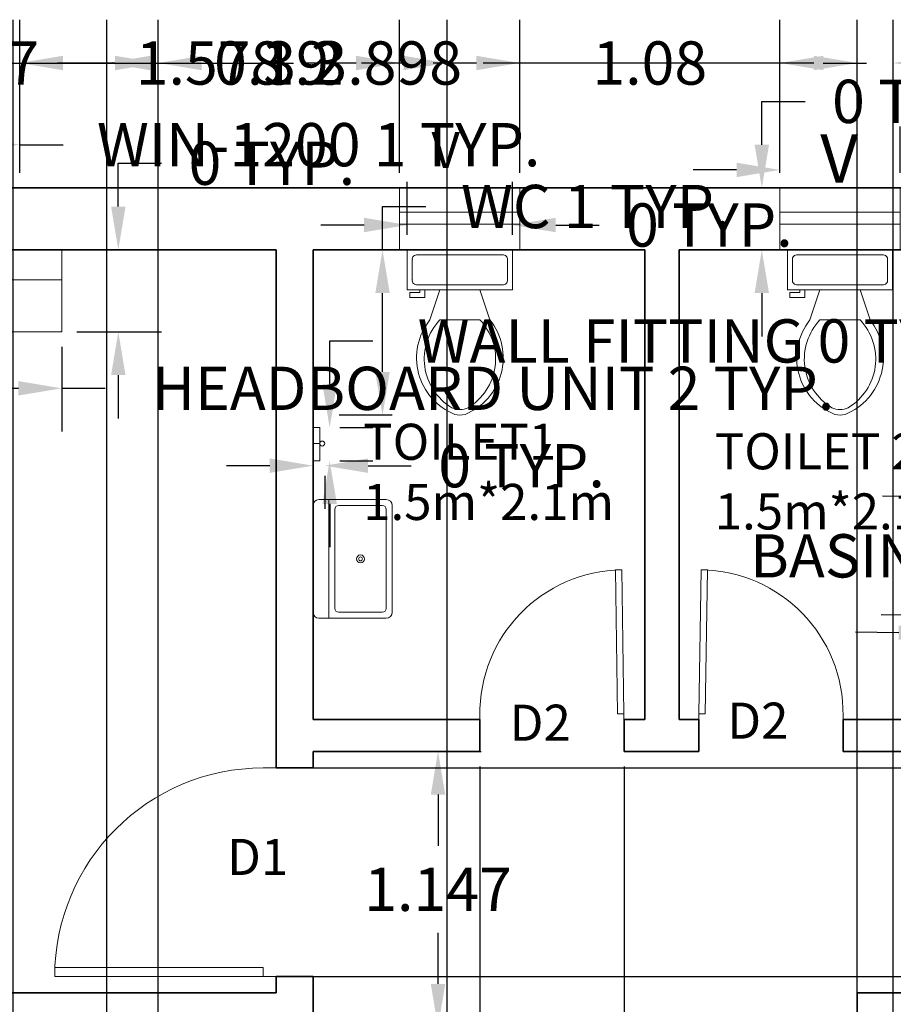
# Model space of a CAD drawing. Units: metres. Extents: x 1988.6 to 2001.1, y 2192 to 2202.5.
# Tile 4 of 6: x 1991.6 to 1995.3, y 2198.4 to 2202.5. Entities that reach past the tile are written whole.
import ezdxf

# ---------------------------------------------------------------- set-up
doc = ezdxf.new("R2010")
doc.units = ezdxf.units.M
for name, color, linetype, lineweight in [('A-ANNO-DIMS', 2, 'Continuous', 18), ('A-ANNO-TEXT', 7, 'Continuous', 18), ('A-AREA-IDEN', 7, 'Continuous', 18), ('A-DOOR', 3, 'Continuous', 18), ('A-FLOR-FIXT', 9, 'Continuous', 18), ('A-FURN', 9, 'Continuous', 15), ('A-GLAZ', 4, 'Continuous', 18), ('A-WALL', 7, 'Continuous', 35)]:
    doc.layers.add(name, color=color, linetype=linetype, lineweight=lineweight)
doc.styles.get("Standard").update_dxf_attribs({"font": 'arial.ttf'})
doc.dimstyles.get("Standard").update_dxf_attribs({"dimtxt": 0.18, "dimasz": 0.18, "dimexe": 0.18, "dimexo": 0.0625, "dimgap": 0.09, "dimtad": 0, "dimtih": 1, "dimtoh": 1, "dimdec": 4, "dimzin": 0, "dimdsep": 46, "dimtxsty": 'Standard', "dimcen": 0.09, "dimadec": 0, "dimazin": 0, "dimtfac": 1, "dimtdec": 4, "dimtofl": 0, "dimtmove": 0, "dimatfit": 3, "dimfxl": 1, "dimtolj": 1, "dimtzin": 0, "dimarcsym": 0})

# ---------------------------------------------------------------- blocks, each defined once
blk = doc.blocks.new('Toilet - top')
for p, q in [((9.5, -6), (9.5, -2)), ((-10, -8.5), (-8, -8.5)), ((-10, -9.5), (-10, -8.5)), ((-7, -9.5), (-10, -9.5)), ((-8, -8.5), (-8, -8)), ((-7, -8), (-7, -9.5)), ((-4, -8), (-6, -14)), ((4, -8), (6, -14)), ((4, -14), (-4, -14))]:
    blk.add_line(p, q)
blk.add_lwpolyline([(10.5, -8), (10.5, 0), (-10.5, 0), (-10.5, -8)], close=True)
for points in [[(8.5, -1), (-8.5, -1)], [(-9.5, -2), (-9.5, -6)], [(-8.5, -7), (8.5, -7)]]:
    blk.add_lwpolyline(points)
for centre, radius, start, end in [((-8.62, -1.88), 0.884, 81.8699, 188.1301), ((8.62, -1.88), 0.884, 351.8699, 98.1301), ((-8.62, -6.12), 0.884, 171.8699, 278.1301), ((8.62, -6.12), 0.884, 261.8699, 8.1301), ((3.52, -21.58), 12.17, 141.4691, 247.9714), ((4.2, -21.82), 11.33, 136.3677, 238.9468), ((-3.52, -21.58), 12.17, 292.0284, 38.5307), ((-4.2, -21.82), 11.33, 301.053, 43.6321), ((0, -27.88), 4, 245.7318, 294.2682), ((0, -29), 4, 254.8605, 285.1395)]:
    blk.add_arc(centre, radius, start, end)
blk = doc.blocks.new('Sink-single - 30 in top')
blk.add_line((-15, -3.999996), (15, -3.999996))
for points in [[(-13.5, 0), (13.5, 0)], [(-15, -18.499996), (-15, -1.5)], [(15, -1.5), (15, -18.499996)], [(-13.5, -17.499996), (-13.5, -6.499996)], [(-12.5, -5.499996), (12.5, -5.499996)], [(13.5, -6.499996), (13.5, -17.499996)], [(12.5, -18.499996), (-12.5, -18.499996)], [(13.5, -19.999996), (-13.5, -19.999996)]]:
    blk.add_lwpolyline(points)
for radius in [1, 0.5]:
    blk.add_circle((0, -11.999996), radius)
for centre, radius, start, end in [((-13.5, -1.5), 1.5, 90, 180), ((13.5, -1.5), 1.5, 0, 90), ((-12.5, -6.499996), 1, 90, 180), ((12.5, -6.499996), 1, 0, 90), ((-13.5, -18.499996), 1.5, 180, 270), ((-12.5, -17.499996), 1, 180, 270), ((12.5, -17.499996), 1, 270, 0), ((13.5, -18.499996), 1.5, 270, 0)]:
    blk.add_arc(centre, radius, start, end)
blk = doc.blocks.new('*U13')
for p, q in [((0, 0), (0, -6)), ((40, 0), (40, -6))]:
    blk.add_line(p, q)
blk.add_lwpolyline([(0, 0), (0, 40), (1.75, 40), (1.75, 0)], close=True)
blk.add_arc((0, 0), 40, 0, 90)
blk = doc.blocks.new('VENT-500')
for p, q in [((-0.0001, 0.2568), (-0.0001, -0.0002)), ((0.4999, 0.2568), (-0.0001, 0.2568)), ((0.4999, -0.0002), (0.4999, 0.2568)), ((0.4999, 0.1568), (-0.0001, 0.1568)), ((-0.0001, 0.1068), (0.4999, 0.1068)), ((-0.0001, -0.0002), (0.4999, -0.0002))]:
    blk.add_line(p, q)
blk = doc.blocks.new('HEADBOARD-WITH-SIDE-TABLES')
for p, q in [((-0.0002, 0.3408), (-0.0002, 0.2164)), ((1.5674, 0.2164), (1.5674, 0.3408)), ((-0.0002, 0.2164), (1.5674, 0.2164)), ((-0.0002, 0.2164), (-0.0002, 0.0002)), ((1.5674, 0.2164), (1.5674, 0.0002)), ((-0.0002, 0.0002), (0.2181, 0.0002)), ((1.5674, 0.0002), (1.3249, 0.0002))]:
    blk.add_line(p, q)
blk = doc.blocks.new('BATH-WALL-FITTING')
for p, q in [((-0.0001, 0.0002), (-0.0001, 0.138)), ((-0.0001, 0.138), (0.028, 0.138)), ((0.028, 0.1375), (0.028, 0.0002)), ((-0.0001, 0.0715), (0.028, 0.0715)), ((0.028, 0.0002), (-0.0001, 0.0002))]:
    blk.add_line(p, q)
blk.add_circle((0.0382, 0.0715), 0.0103)
blk = doc.blocks.new('*D26')
at = {"layer": 'A-ANNO-DIMS', "color": 0, "lineweight": -2, "transparency": 16777216}
for p, q in [((1993.1277, 2201.4968), (1993.1277, 2201.6768)), ((1993.1277, 2201.6768), (1993.3077, 2201.6768)), ((1993.1683, 2201.4968), (1992.9477, 2201.4968)), ((1993.1277, 2200.9889), (1993.1277, 2201.3168)), ((1993.1683, 2200.8089), (1992.9477, 2200.8089))]:
    blk.add_line(p, q, dxfattribs=at)
at = {"layer": 'A-ANNO-DIMS', "color": 0, "transparency": 16777216}
for points in [[(1993.0977, 2201.3168), (1993.1577, 2201.3168), (1993.1277, 2201.4968)], [(1993.0977, 2200.9889), (1993.1577, 2200.9889), (1993.1277, 2200.8089)]]:
    blk.add_solid(points, dxfattribs=at)
at = {"layer": 'Defpoints', "color": 0, "transparency": 16777216}
for p in [(1993.1277, 2201.4968), (1993.2308, 2201.4968), (1993.2308, 2200.8089)]:
    blk.add_point(p, dxfattribs=at)
at = {"layer": 'A-ANNO-DIMS', "color": 0, "transparency": 16777216, "insert": (1994.0139, 2201.6768), "char_height": 0.18, "attachment_point": 5}
blk.add_mtext('\\A1;WC 1 TYP.', dxfattribs=at)
blk = doc.blocks.new('*D27')
at = {"layer": 'A-ANNO-DIMS', "color": 0, "lineweight": -2, "transparency": 16777216}
for p, q in [((1993.2308, 2201.5593), (1993.2308, 2201.7799)), ((1993.6679, 2201.5593), (1993.6679, 2201.7799)), ((1993.0508, 2201.5999), (1992.8708, 2201.5999)), ((1993.8479, 2201.5999), (1994.0279, 2201.5999))]:
    blk.add_line(p, q, dxfattribs=at)
at = {"layer": 'A-ANNO-DIMS', "color": 0, "transparency": 16777216}
for points in [[(1993.0508, 2201.6299), (1993.0508, 2201.5699), (1993.2308, 2201.5999)], [(1993.8479, 2201.6299), (1993.8479, 2201.5699), (1993.6679, 2201.5999)]]:
    blk.add_solid(points, dxfattribs=at)
at = {"layer": 'Defpoints', "color": 0, "transparency": 16777216}
for p in [(1993.6679, 2201.5999), (1993.2308, 2201.4968), (1993.6679, 2201.4968)]:
    blk.add_point(p, dxfattribs=at)
at = {"layer": 'A-ANNO-DIMS', "color": 0, "transparency": 16777216, "insert": (1994.4861, 2201.5999), "char_height": 0.18, "attachment_point": 5}
blk.add_mtext('\\A1;0 TYP.', dxfattribs=at)
blk = doc.blocks.new('*D28')
at = {"layer": 'A-ANNO-DIMS', "color": 0, "lineweight": -2, "transparency": 16777216}
for p, q in [((1995.3871, 2200.6513), (1995.3891, 2200.8313)), ((1995.3967, 2200.4712), (1995.2052, 2200.4733)), ((1995.3914, 2199.9779), (1995.1999, 2199.98)), ((1995.3779, 2199.7981), (1995.376, 2199.6181))]:
    blk.add_line(p, q, dxfattribs=at)
at = {"layer": 'A-ANNO-DIMS', "color": 0, "transparency": 16777216}
for points in [[(1995.3571, 2200.6517), (1995.4171, 2200.651), (1995.3852, 2200.4714)], [(1995.3479, 2199.7984), (1995.4079, 2199.7978), (1995.3799, 2199.9781)]]:
    blk.add_solid(points, dxfattribs=at)
at = {"layer": 'Defpoints', "color": 0, "transparency": 16777216}
for p in [(1995.4592, 2200.4706), (1995.3799, 2199.9781), (1995.4538, 2199.9773)]:
    blk.add_point(p, dxfattribs=at)
at = {"layer": 'A-ANNO-DIMS', "color": 0, "transparency": 16777216, "insert": (1995.3825, 2200.2247), "char_height": 0.18, "attachment_point": 5}
blk.add_mtext('\\A1;BASIN 0 TYP.', dxfattribs=at)
blk = doc.blocks.new('*D29')
at = {"layer": 'A-ANNO-DIMS', "color": 0, "lineweight": -2, "transparency": 16777216}
for p, q in [((1995.2731, 2199.9052), (1995.0931, 2199.9072)), ((1995.4532, 2199.9148), (1995.4511, 2199.7233)), ((1995.782, 2199.9112), (1995.78, 2199.7197)), ((1995.9619, 2199.8978), (1996.1419, 2199.8958))]:
    blk.add_line(p, q, dxfattribs=at)
at = {"layer": 'A-ANNO-DIMS', "color": 0, "transparency": 16777216}
for points in [[(1995.2734, 2199.9352), (1995.2727, 2199.8752), (1995.453, 2199.9033)], [(1995.9622, 2199.9278), (1995.9616, 2199.8678), (1995.7819, 2199.8997)]]:
    blk.add_solid(points, dxfattribs=at)
at = {"layer": 'Defpoints', "color": 0, "transparency": 16777216}
for p in [(1995.4538, 2199.9773), (1995.7827, 2199.9737), (1995.7819, 2199.8997)]:
    blk.add_point(p, dxfattribs=at)
at = {"layer": 'A-ANNO-DIMS', "color": 0, "transparency": 16777216, "insert": (1996.6, 2199.8958), "char_height": 0.18, "attachment_point": 5}
blk.add_mtext('\\A1;0 TYP.', dxfattribs=at)
blk = doc.blocks.new('*D32')
at = {"layer": 'A-ANNO-DIMS', "color": 0, "lineweight": -2, "transparency": 16777216}
for p, q in [((1990.4198, 2201.8163), (1990.4198, 2202.1138)), ((1991.6198, 2201.8163), (1991.6198, 2202.1138)), ((1990.5998, 2201.9338), (1991.4398, 2201.9338)), ((1991.6198, 2201.9338), (1991.7998, 2201.9338))]:
    blk.add_line(p, q, dxfattribs=at)
at = {"layer": 'A-ANNO-DIMS', "color": 0, "transparency": 16777216}
for points in [[(1990.5998, 2201.9638), (1990.5998, 2201.9038), (1990.4198, 2201.9338)], [(1991.4398, 2201.9638), (1991.4398, 2201.9038), (1991.6198, 2201.9338)]]:
    blk.add_solid(points, dxfattribs=at)
at = {"layer": 'Defpoints', "color": 0, "transparency": 16777216}
for p in [(1991.6198, 2201.9338), (1990.4198, 2201.7538), (1991.6198, 2201.7538)]:
    blk.add_point(p, dxfattribs=at)
at = {"layer": 'A-ANNO-DIMS', "color": 0, "transparency": 16777216, "insert": (1992.8625, 2201.9338), "char_height": 0.18, "attachment_point": 5}
blk.add_mtext('\\A1;WIN-1200 1 TYP.', dxfattribs=at)
blk = doc.blocks.new('*D34')
at = {"layer": 'A-ANNO-DIMS', "color": 0, "lineweight": -2, "transparency": 16777216}
for p, q in [((1994.7792, 2201.8163), (1994.7792, 2202.0088)), ((1995.2792, 2201.8163), (1995.2792, 2202.0088)), ((1994.5992, 2201.8288), (1994.4192, 2201.8288)), ((1995.4592, 2201.8288), (1995.6392, 2201.8288))]:
    blk.add_line(p, q, dxfattribs=at)
at = {"layer": 'A-ANNO-DIMS', "color": 0, "transparency": 16777216}
for points in [[(1994.5992, 2201.8588), (1994.5992, 2201.7988), (1994.7792, 2201.8288)], [(1995.4592, 2201.8588), (1995.4592, 2201.7988), (1995.2792, 2201.8288)]]:
    blk.add_solid(points, dxfattribs=at)
at = {"layer": 'Defpoints', "color": 0, "transparency": 16777216}
for p in [(1995.2792, 2201.8288), (1994.7792, 2201.7538), (1995.2792, 2201.7538)]:
    blk.add_point(p, dxfattribs=at)
at = {"layer": 'A-ANNO-DIMS', "color": 0, "transparency": 16777216, "insert": (1996.724, 2201.8288), "char_height": 0.18, "attachment_point": 5}
blk.add_mtext('\\A1;VENT-500 1 TYP.', dxfattribs=at)
blk = doc.blocks.new('*D35')
at = {"layer": 'A-ANNO-DIMS', "color": 0, "lineweight": -2, "transparency": 16777216}
for p, q in [((1994.7042, 2201.9338), (1994.7042, 2202.1138)), ((1994.7042, 2202.1138), (1994.8842, 2202.1138)), ((1994.7167, 2201.7538), (1994.5242, 2201.7538)), ((1994.7167, 2201.4968), (1994.5242, 2201.4968)), ((1994.7042, 2201.3168), (1994.7042, 2201.1368))]:
    blk.add_line(p, q, dxfattribs=at)
at = {"layer": 'A-ANNO-DIMS', "color": 0, "transparency": 16777216}
for points in [[(1994.6742, 2201.9338), (1994.7342, 2201.9338), (1994.7042, 2201.7538)], [(1994.6742, 2201.3168), (1994.7342, 2201.3168), (1994.7042, 2201.4968)]]:
    blk.add_solid(points, dxfattribs=at)
at = {"layer": 'Defpoints', "color": 0, "transparency": 16777216}
for p in [(1994.7042, 2201.7538), (1994.7792, 2201.7538), (1994.7792, 2201.4968)]:
    blk.add_point(p, dxfattribs=at)
at = {"layer": 'A-ANNO-DIMS', "color": 0, "transparency": 16777216, "insert": (1995.3424, 2202.1138), "char_height": 0.18, "attachment_point": 5}
blk.add_mtext('\\A1;0 TYP.', dxfattribs=at)
blk = doc.blocks.new('*D36')
at = {"layer": 'A-ANNO-DIMS', "color": 0, "lineweight": -2, "transparency": 16777216}
for p, q in [((1990.2268, 2201.0937), (1990.2268, 2200.741)), ((1991.7944, 2201.0937), (1991.7944, 2200.741)), ((1990.4068, 2200.921), (1991.6144, 2200.921)), ((1991.7944, 2200.921), (1991.9744, 2200.921))]:
    blk.add_line(p, q, dxfattribs=at)
at = {"layer": 'A-ANNO-DIMS', "color": 0, "transparency": 16777216}
for points in [[(1990.4068, 2200.951), (1990.4068, 2200.891), (1990.2268, 2200.921)], [(1991.6144, 2200.951), (1991.6144, 2200.891), (1991.7944, 2200.921)]]:
    blk.add_solid(points, dxfattribs=at)
at = {"layer": 'Defpoints', "color": 0, "transparency": 16777216}
for p in [(1990.2268, 2201.1562), (1991.7944, 2201.1562), (1991.7944, 2200.921)]:
    blk.add_point(p, dxfattribs=at)
at = {"layer": 'A-ANNO-DIMS', "color": 0, "transparency": 16777216, "insert": (1993.5874, 2200.921), "char_height": 0.18, "attachment_point": 5}
blk.add_mtext('\\A1;HEADBOARD UNIT 2 TYP.', dxfattribs=at)
blk = doc.blocks.new('*D37')
at = {"layer": 'A-ANNO-DIMS', "color": 0, "lineweight": -2, "transparency": 16777216}
for p, q in [((1992.0296, 2201.6768), (1992.0296, 2201.8568)), ((1992.0296, 2201.8568), (1992.2096, 2201.8568)), ((1991.8569, 2201.4968), (1992.2096, 2201.4968)), ((1991.8569, 2201.1562), (1992.2096, 2201.1562)), ((1992.0296, 2200.9762), (1992.0296, 2200.7962))]:
    blk.add_line(p, q, dxfattribs=at)
at = {"layer": 'A-ANNO-DIMS', "color": 0, "transparency": 16777216}
for points in [[(1991.9996, 2201.6768), (1992.0596, 2201.6768), (1992.0296, 2201.4968)], [(1991.9996, 2200.9762), (1992.0596, 2200.9762), (1992.0296, 2201.1562)]]:
    blk.add_solid(points, dxfattribs=at)
at = {"layer": 'Defpoints', "color": 0, "transparency": 16777216}
for p in [(1991.7944, 2201.4968), (1992.0296, 2201.4968), (1991.7944, 2201.1562)]:
    blk.add_point(p, dxfattribs=at)
at = {"layer": 'A-ANNO-DIMS', "color": 0, "transparency": 16777216, "insert": (1992.6677, 2201.8568), "char_height": 0.18, "attachment_point": 5}
blk.add_mtext('\\A1;0 TYP.', dxfattribs=at)
blk = doc.blocks.new('*D42')
at = {"layer": 'A-ANNO-DIMS', "color": 0, "lineweight": -2, "transparency": 16777216}
for p, q in [((1992.9081, 2200.938), (1992.9081, 2201.118)), ((1992.9081, 2201.118), (1993.0881, 2201.118)), ((1992.95, 2200.758), (1993.0881, 2200.758)), ((1992.95, 2200.6202), (1993.0881, 2200.6202)), ((1992.9081, 2200.4402), (1992.9081, 2200.2602))]:
    blk.add_line(p, q, dxfattribs=at)
at = {"layer": 'A-ANNO-DIMS', "color": 0, "transparency": 16777216}
for points in [[(1992.8781, 2200.938), (1992.9381, 2200.938), (1992.9081, 2200.758)], [(1992.8781, 2200.4402), (1992.9381, 2200.4402), (1992.9081, 2200.6202)]]:
    blk.add_solid(points, dxfattribs=at)
at = {"layer": 'Defpoints', "color": 0, "transparency": 16777216}
for p in [(1992.8875, 2200.758), (1992.9081, 2200.758), (1992.8875, 2200.6202)]:
    blk.add_point(p, dxfattribs=at)
at = {"layer": 'A-ANNO-DIMS', "color": 0, "transparency": 16777216, "insert": (1994.4511, 2201.118), "char_height": 0.18, "attachment_point": 5}
blk.add_mtext('\\A1;WALL FITTING 0 TYP.', dxfattribs=at)
blk = doc.blocks.new('*D43')
at = {"layer": 'A-ANNO-DIMS', "color": 0, "lineweight": -2, "transparency": 16777216}
for p, q in [((1992.6589, 2200.5995), (1992.4789, 2200.5995)), ((1993.0675, 2200.5995), (1993.2475, 2200.5995)), ((1992.8389, 2200.5577), (1992.8389, 2200.4195)), ((1992.8875, 2200.5577), (1992.8875, 2200.4195))]:
    blk.add_line(p, q, dxfattribs=at)
at = {"layer": 'A-ANNO-DIMS', "color": 0, "transparency": 16777216}
for points in [[(1992.6589, 2200.6295), (1992.6589, 2200.5695), (1992.8389, 2200.5995)], [(1993.0675, 2200.6295), (1993.0675, 2200.5695), (1992.8875, 2200.5995)]]:
    blk.add_solid(points, dxfattribs=at)
at = {"layer": 'Defpoints', "color": 0, "transparency": 16777216}
for p in [(1992.8389, 2200.6202), (1992.8875, 2200.6202), (1992.8875, 2200.5995)]:
    blk.add_point(p, dxfattribs=at)
at = {"layer": 'A-ANNO-DIMS', "color": 0, "transparency": 16777216, "insert": (1993.7056, 2200.5995), "char_height": 0.18, "attachment_point": 5}
blk.add_mtext('\\A1;0 TYP.', dxfattribs=at)
blk = doc.blocks.new('*D55')
at = {"layer": 'A-ANNO-DIMS', "color": 0, "lineweight": -2, "transparency": 16777216}
for p, q in [((1991.6198, 2201.8163), (1991.6198, 2202.4533)), ((1993.1979, 2201.8163), (1993.1979, 2202.4533)), ((1991.7998, 2202.2733), (1992.0234, 2202.2733)), ((1993.0179, 2202.2733), (1992.7942, 2202.2733))]:
    blk.add_line(p, q, dxfattribs=at)
at = {"layer": 'A-ANNO-DIMS', "color": 0, "transparency": 16777216}
for points in [[(1991.7998, 2202.3033), (1991.7998, 2202.2433), (1991.6198, 2202.2733)], [(1993.0179, 2202.3033), (1993.0179, 2202.2433), (1993.1979, 2202.2733)]]:
    blk.add_solid(points, dxfattribs=at)
at = {"layer": 'Defpoints', "color": 0, "transparency": 16777216}
for p in [(1993.1979, 2202.2733), (1991.6198, 2201.7538), (1993.1979, 2201.7538)]:
    blk.add_point(p, dxfattribs=at)
at = {"layer": 'A-ANNO-DIMS', "color": 0, "transparency": 16777216, "insert": (1992.4088, 2202.2733), "char_height": 0.18, "attachment_point": 5}
blk.add_mtext('\\A1;1.578', dxfattribs=at)
blk = doc.blocks.new('*D56')
at = {"layer": 'A-ANNO-DIMS', "color": 0, "lineweight": -2, "transparency": 16777216}
for p, q in [((1993.6979, 2201.8163), (1993.6979, 2202.4533)), ((1994.7792, 2201.8163), (1994.7792, 2202.4533)), ((1993.5179, 2202.2733), (1993.3379, 2202.2733)), ((1994.9592, 2202.2733), (1995.1392, 2202.2733))]:
    blk.add_line(p, q, dxfattribs=at)
at = {"layer": 'A-ANNO-DIMS', "color": 0, "transparency": 16777216}
for points in [[(1993.5179, 2202.3033), (1993.5179, 2202.2433), (1993.6979, 2202.2733)], [(1994.9592, 2202.3033), (1994.9592, 2202.2433), (1994.7792, 2202.2733)]]:
    blk.add_solid(points, dxfattribs=at)
at = {"layer": 'Defpoints', "color": 0, "transparency": 16777216}
for p in [(1994.7792, 2202.2733), (1993.6979, 2201.7538), (1994.7792, 2201.7538)]:
    blk.add_point(p, dxfattribs=at)
at = {"layer": 'A-ANNO-DIMS', "color": 0, "transparency": 16777216, "insert": (1994.2386, 2202.2733), "char_height": 0.18, "attachment_point": 5}
blk.add_mtext('\\A1;1.08', dxfattribs=at)
blk = doc.blocks.new('*D60')
at = {"layer": 'A-ANNO-DIMS', "color": 0, "lineweight": -2, "transparency": 16777216}
for p, q in [((1990.7282, 2193.0163), (1990.7282, 2202.4533)), ((1992.1958, 2193.0163), (1992.1958, 2202.4533)), ((1990.9082, 2202.2733), (1991.1467, 2202.2733)), ((1992.0158, 2202.2733), (1991.7773, 2202.2733))]:
    blk.add_line(p, q, dxfattribs=at)
at = {"layer": 'A-ANNO-DIMS', "color": 0, "transparency": 16777216}
for points in [[(1990.9082, 2202.3033), (1990.9082, 2202.2433), (1990.7282, 2202.2733)], [(1992.0158, 2202.3033), (1992.0158, 2202.2433), (1992.1958, 2202.2733)]]:
    blk.add_solid(points, dxfattribs=at)
at = {"layer": 'Defpoints', "color": 0, "transparency": 16777216}
for p in [(1992.1958, 2202.2733), (1990.7282, 2192.9538), (1992.1958, 2192.9538)]:
    blk.add_point(p, dxfattribs=at)
at = {"layer": 'A-ANNO-DIMS', "color": 0, "transparency": 16777216, "insert": (1991.462, 2202.2733), "char_height": 0.18, "attachment_point": 5}
blk.add_mtext('\\A1;1.47', dxfattribs=at)
blk = doc.blocks.new('*D61')
at = {"layer": 'A-ANNO-DIMS', "color": 0, "lineweight": -2, "transparency": 16777216}
for p, q in [((1992.1958, 2193.0163), (1992.1958, 2202.4533)), ((1993.3958, 2193.0163), (1993.3958, 2202.4533)), ((1992.3758, 2202.2733), (1992.5513, 2202.2733)), ((1993.2158, 2202.2733), (1993.0402, 2202.2733))]:
    blk.add_line(p, q, dxfattribs=at)
at = {"layer": 'A-ANNO-DIMS', "color": 0, "transparency": 16777216}
for points in [[(1992.3758, 2202.3033), (1992.3758, 2202.2433), (1992.1958, 2202.2733)], [(1993.2158, 2202.3033), (1993.2158, 2202.2433), (1993.3958, 2202.2733)]]:
    blk.add_solid(points, dxfattribs=at)
at = {"layer": 'Defpoints', "color": 0, "transparency": 16777216}
for p in [(1993.3958, 2202.2733), (1992.1958, 2192.9538), (1993.3958, 2192.9538)]:
    blk.add_point(p, dxfattribs=at)
at = {"layer": 'A-ANNO-DIMS', "color": 0, "transparency": 16777216, "insert": (1992.7958, 2202.2733), "char_height": 0.18, "attachment_point": 5}
blk.add_mtext('\\A1;1.2', dxfattribs=at)
blk = doc.blocks.new('*D63')
at = {"layer": 'A-ANNO-DIMS', "color": 0, "lineweight": -2, "transparency": 16777216}
for p, q in [((1991.2026, 2195.283), (1991.2026, 2202.4533)), ((1995.1007, 2195.283), (1995.1007, 2202.4533)), ((1991.3826, 2202.2733), (1992.7578, 2202.2733)), ((1994.9207, 2202.2733), (1993.5455, 2202.2733))]:
    blk.add_line(p, q, dxfattribs=at)
at = {"layer": 'A-ANNO-DIMS', "color": 0, "transparency": 16777216}
for points in [[(1991.3826, 2202.3033), (1991.3826, 2202.2433), (1991.2026, 2202.2733)], [(1994.9207, 2202.3033), (1994.9207, 2202.2433), (1995.1007, 2202.2733)]]:
    blk.add_solid(points, dxfattribs=at)
at = {"layer": 'Defpoints', "color": 0, "transparency": 16777216}
for p in [(1995.1007, 2202.2733), (1991.2026, 2195.2205), (1995.1007, 2195.2205)]:
    blk.add_point(p, dxfattribs=at)
at = {"layer": 'A-ANNO-DIMS', "color": 0, "transparency": 16777216, "insert": (1993.1516, 2202.2733), "char_height": 0.18, "attachment_point": 5}
blk.add_mtext('\\A1;3.898', dxfattribs=at)
blk = doc.blocks.new('*D67')
at = {"layer": 'A-ANNO-DIMS', "color": 0, "lineweight": -2, "transparency": 16777216}
for p, q in [((1991.5924, 2194.3163), (1991.5924, 2202.4533)), ((1991.9822, 2194.3163), (1991.9822, 2202.4533)), ((1991.4124, 2202.2733), (1991.2324, 2202.2733)), ((1992.1622, 2202.2733), (1992.3422, 2202.2733))]:
    blk.add_line(p, q, dxfattribs=at)
at = {"layer": 'A-ANNO-DIMS', "color": 0, "transparency": 16777216}
for points in [[(1991.4124, 2202.3033), (1991.4124, 2202.2433), (1991.5924, 2202.2733)], [(1992.1622, 2202.3033), (1992.1622, 2202.2433), (1991.9822, 2202.2733)]]:
    blk.add_solid(points, dxfattribs=at)
at = {"layer": 'Defpoints', "color": 0, "transparency": 16777216}
for p in [(1991.9822, 2202.2733), (1991.5924, 2194.2538), (1991.9822, 2194.2538)]:
    blk.add_point(p, dxfattribs=at)
at = {"layer": 'A-ANNO-DIMS', "color": 0, "transparency": 16777216, "insert": (1992.6662, 2202.2733), "char_height": 0.18, "attachment_point": 5}
blk.add_mtext('\\A1;0.39', dxfattribs=at)
blk = doc.blocks.new('*D72')
at = {"layer": 'A-ANNO-DIMS', "color": 0, "lineweight": -2, "transparency": 16777216}
for p, q in [((1999.9013, 2199.3431), (1999.9013, 2199.5231)), ((1999.9013, 2199.5231), (2000.0813, 2199.5231)), ((1992.7483, 2199.3431), (2000.0813, 2199.3431)), ((1999.9013, 2198.656), (1999.9013, 2199.1631)), ((1992.7483, 2198.476), (2000.0813, 2198.476))]:
    blk.add_line(p, q, dxfattribs=at)
at = {"layer": 'A-ANNO-DIMS', "color": 0, "transparency": 16777216}
for points in [[(1999.8713, 2199.1631), (1999.9313, 2199.1631), (1999.9013, 2199.3431)], [(1999.8713, 2198.656), (1999.9313, 2198.656), (1999.9013, 2198.476)]]:
    blk.add_solid(points, dxfattribs=at)
at = {"layer": 'Defpoints', "color": 0, "transparency": 16777216}
for p in [(1992.6858, 2199.3431), (1999.9013, 2199.3431), (1992.6858, 2198.476)]:
    blk.add_point(p, dxfattribs=at)
at = {"layer": 'A-ANNO-DIMS', "color": 0, "transparency": 16777216, "insert": (2000.4051, 2199.5231), "char_height": 0.18, "attachment_point": 5}
blk.add_mtext('\\A1;0.87', dxfattribs=at)
blk = doc.blocks.new('*D73')
at = {"layer": 'A-ANNO-DIMS', "color": 0, "lineweight": -2, "transparency": 16777216}
for p, q in [((1993.5324, 2199.3495), (1993.5324, 2192.0043)), ((1994.1324, 2199.3495), (1994.1324, 2192.0043)), ((1993.7124, 2192.1843), (1993.9524, 2192.1843)), ((1994.1324, 2192.1843), (1994.3124, 2192.1843))]:
    blk.add_line(p, q, dxfattribs=at)
at = {"layer": 'A-ANNO-DIMS', "color": 0, "transparency": 16777216}
for points in [[(1993.7124, 2192.2143), (1993.7124, 2192.1543), (1993.5324, 2192.1843)], [(1993.9524, 2192.2143), (1993.9524, 2192.1543), (1994.1324, 2192.1843)]]:
    blk.add_solid(points, dxfattribs=at)
at = {"layer": 'Defpoints', "color": 0, "transparency": 16777216}
for p in [(1993.5324, 2199.412), (1994.1324, 2199.412), (1994.1324, 2192.1843)]:
    blk.add_point(p, dxfattribs=at)
at = {"layer": 'A-ANNO-DIMS', "color": 0, "transparency": 16777216, "insert": (1994.5662, 2192.1843), "char_height": 0.18, "attachment_point": 5}
blk.add_mtext('\\A1;0.6', dxfattribs=at)
blk = doc.blocks.new('*D75')
at = {"layer": 'A-ANNO-DIMS', "color": 0, "lineweight": -2, "transparency": 16777216}
for p, q in [((1995.1007, 2198.4713), (1995.1007, 2202.4533)), ((1995.2507, 2198.3276), (1995.2507, 2202.4533)), ((1994.9207, 2202.2733), (1994.7407, 2202.2733)), ((1995.4307, 2202.2733), (1995.6107, 2202.2733))]:
    blk.add_line(p, q, dxfattribs=at)
at = {"layer": 'A-ANNO-DIMS', "color": 0, "transparency": 16777216}
for points in [[(1994.9207, 2202.3033), (1994.9207, 2202.2433), (1995.1007, 2202.2733)], [(1995.4307, 2202.3033), (1995.4307, 2202.2433), (1995.2507, 2202.2733)]]:
    blk.add_solid(points, dxfattribs=at)
at = {"layer": 'Defpoints', "color": 0, "transparency": 16777216}
for p in [(1995.2507, 2202.2733), (1995.1007, 2198.4088), (1995.2507, 2198.2651)]:
    blk.add_point(p, dxfattribs=at)
at = {"layer": 'A-ANNO-DIMS', "color": 0, "transparency": 16777216, "insert": (1995.9351, 2202.2733), "char_height": 0.18, "attachment_point": 5}
blk.add_mtext('\\A1;0.15', dxfattribs=at)
blk = doc.blocks.new('*D79')
at = {"layer": 'A-ANNO-DIMS', "color": 0, "lineweight": -2, "transparency": 16777216}
for p, q in [((1992.9014, 2199.412), (1993.5384, 2199.412)), ((1993.3584, 2199.232), (1993.3584, 2199.0189)), ((1993.3584, 2198.4451), (1993.3584, 2198.6581)), ((1992.9014, 2198.2651), (1993.5384, 2198.2651))]:
    blk.add_line(p, q, dxfattribs=at)
at = {"layer": 'A-ANNO-DIMS', "color": 0, "transparency": 16777216}
for points in [[(1993.3284, 2199.232), (1993.3884, 2199.232), (1993.3584, 2199.412)], [(1993.3284, 2198.4451), (1993.3884, 2198.4451), (1993.3584, 2198.2651)]]:
    blk.add_solid(points, dxfattribs=at)
at = {"layer": 'Defpoints', "color": 0, "transparency": 16777216}
for p in [(1992.8389, 2199.412), (1992.8389, 2198.2651), (1993.3584, 2198.2651)]:
    blk.add_point(p, dxfattribs=at)
at = {"layer": 'A-ANNO-DIMS', "color": 0, "transparency": 16777216, "insert": (1993.3584, 2198.8385), "char_height": 0.18, "attachment_point": 5}
blk.add_mtext('\\A1;1.147', dxfattribs=at)

msp = doc.modelspace()

# ---------------------------------------------------------------- linework, layer by layer
at = {"layer": 'A-WALL'}
for p, q in [((1999.3818, 2201.7538), (1989.3818, 2201.7538)), ((1992.6858, 2201.4968), (1989.6351, 2201.4968)), ((1992.6858, 2201.4968), (1992.6858, 2199.3431)), ((1992.8389, 2201.4968), (1992.8389, 2199.545)), ((1994.2178, 2201.4968), (1992.8389, 2201.4968)), ((1994.2178, 2201.4968), (1994.2178, 2199.545)), ((1994.36, 2201.4968), (1994.36, 2199.545)), ((1995.7849, 2201.4968), (1994.36, 2201.4968)), ((1993.5324, 2199.545), (1992.8389, 2199.545)), ((1993.5324, 2199.545), (1993.5324, 2199.412)), ((1994.2178, 2199.545), (1994.1324, 2199.545)), ((1994.1324, 2199.545), (1994.1324, 2199.412)), ((1994.4418, 2199.545), (1994.36, 2199.545)), ((1994.4418, 2199.545), (1994.4418, 2199.412)), ((1995.7849, 2199.545), (1995.0418, 2199.545)), ((1995.0418, 2199.545), (1995.0418, 2199.412)), ((1992.8389, 2199.412), (1992.8389, 2199.3431)), ((1993.5324, 2199.412), (1992.8389, 2199.412)), ((1994.4418, 2199.412), (1994.1324, 2199.412)), ((1995.7849, 2199.412), (1995.0418, 2199.412)), ((1992.6858, 2199.3431), (1992.8389, 2199.3431)), ((1992.6858, 2198.476), (1992.8389, 2198.476)), ((1992.6858, 2198.476), (1992.6858, 2198.4088)), ((1992.8389, 2198.476), (1992.8389, 2198.2651)), ((1992.6858, 2198.4088), (1989.6351, 2198.4088)), ((1995.7849, 2198.4088), (1995.1007, 2198.4088)), ((1995.1007, 2197.698), (1995.1007, 2198.4088))]:
    msp.add_line(p, q, dxfattribs=at)

# ---------------------------------------------------------------- block references
at = {"layer": 'A-DOOR'}
for p, xscale, yscale, zscale, rotation in [((1994.1311, 2199.5683), -0.0149691911654328, 0.0149691911654328, 0.0149691911654328, 0.8479922566477603), ((1994.4431, 2199.5683), 0.0149691911654328, 0.0149691911654328, 0.0149691911654328, 359.1520077433523), ((1992.6323, 2198.476), 0.021677520635372, 0.021677520635372, 0.021677520635372, 90)]:
    msp.add_blockref('*U13', p, dxfattribs=dict(at, xscale=xscale, yscale=yscale, zscale=zscale, rotation=rotation))
at = {"layer": 'A-FLOR-FIXT', "xscale": 0.0208149819866856, "yscale": 0.0208149819866856, "zscale": 0.0208149819866856}
for p in [(1993.4494, 2201.4968), (1995.0292, 2201.4968)]:
    msp.add_blockref('Toilet - top', p, dxfattribs=at)
at = {"layer": 'A-FLOR-FIXT'}
msp.add_blockref('BATH-WALL-FITTING', (1992.839, 2200.62), dxfattribs=at)
at = {"layer": 'A-FLOR-FIXT', "xscale": 0.0164438288540887, "yscale": 0.0164438288540887, "zscale": 0.0164438288540887, "rotation": 90}
msp.add_blockref('Sink-single - 30 in top', (1992.8389, 2200.212), dxfattribs=at)
at = {"layer": 'A-FURN'}
msp.add_blockref('HEADBOARD-WITH-SIDE-TABLES', (1990.227, 2201.156), dxfattribs=at)
at = {"layer": 'A-GLAZ'}
for p in [(1993.198, 2201.497), (1994.7794, 2201.497)]:
    msp.add_blockref('VENT-500', p, dxfattribs=at)

# ---------------------------------------------------------------- texts
at = {"layer": 'A-ANNO-TEXT', "attachment_point": 1}
for s, insert, char_height in [('V', (1993.3313, 2201.9866), 0.15), ('V', (1994.9473, 2201.9762), 0.2), ('D2', (1993.656, 2199.606), 0.15), ('D2  ', (1994.5605, 2199.6145), 0.15), ('D1', (1992.4814, 2199.048), 0.15)]:
    msp.add_mtext_dynamic_manual_height_columns(s, width=0.386628, gutter_width=12.5, heights=[0], dxfattribs=dict(at, insert=insert, char_height=char_height))
at = {"layer": 'A-AREA-IDEN', "char_height": 0.15, "attachment_point": 1}
for s, insert in [('TOILET1\\P1.5m*2.1m', (1993.0474, 2200.7738)), ('TOILET 2\\P1.5m*2.1m', (1994.5087, 2200.7343))]:
    msp.add_mtext_dynamic_manual_height_columns(s, width=1.378048, gutter_width=12.5, heights=[0], dxfattribs=dict(at, insert=insert))

# ---------------------------------------------------------------- dimensions: what is measured, and where the dimension line sits
at = {"layer": 'A-ANNO-DIMS'}
for base, p1, p2, override, picture, middle in [((1992.1958, 2202.2733), (1990.7282, 2192.9538), (1992.1958, 2192.9538), {"dimdec": 2, "dimlfac": 1, "dimrnd": 0, "dimzin": 0, "dimdsep": 46, "dimlunit": 2}, '*D60', (1991.462, 2202.2733)), ((1995.1007, 2202.2733), (1991.2026, 2195.2205), (1995.1007, 2195.2205), {"dimdec": 3, "dimlfac": 1, "dimrnd": 0, "dimzin": 0, "dimdsep": 46, "dimlunit": 2}, '*D63', (1993.1516, 2202.2733)), ((1991.9822, 2202.2733), (1991.5924, 2194.2538), (1991.9822, 2194.2538), {"dimdec": 2, "dimlfac": 1, "dimrnd": 0, "dimzin": 0, "dimdsep": 46, "dimlunit": 2}, '*D67', (1992.6662, 2202.2733)), ((1993.1979, 2202.2733), (1991.6198, 2201.7538), (1993.1979, 2201.7538), {"dimdec": 3, "dimlfac": 1, "dimrnd": 0, "dimzin": 0, "dimdsep": 46, "dimlunit": 2}, '*D55', (1992.4088, 2202.2733)), ((1993.3958, 2202.2733), (1992.1958, 2192.9538), (1993.3958, 2192.9538), {"dimdec": 1, "dimlfac": 1, "dimrnd": 0, "dimzin": 0, "dimdsep": 46, "dimlunit": 2}, '*D61', (1992.7958, 2202.2733)), ((1994.7792, 2202.2733), (1993.6979, 2201.7538), (1994.7792, 2201.7538), {"dimdec": 2, "dimlfac": 1, "dimrnd": 0, "dimzin": 0, "dimdsep": 46, "dimlunit": 2}, '*D56', (1994.2386, 2202.2733)), ((1995.2507, 2202.2733), (1995.1007, 2198.4088), (1995.2507, 2198.2651), {"dimdec": 2, "dimlfac": 1, "dimrnd": 0, "dimzin": 0, "dimdsep": 46, "dimlunit": 2}, '*D75', (1995.9351, 2202.2733)), ((1994.1324, 2192.1843), (1993.5324, 2199.412), (1994.1324, 2199.412), {"dimdec": 1, "dimlfac": 1, "dimrnd": 0, "dimzin": 0, "dimdsep": 46, "dimlunit": 2}, '*D73', (1994.5662, 2192.1843))]:
    dim = msp.add_linear_dim(base=base, p1=p1, p2=p2, dimstyle='Standard', override=override, dxfattribs=at)
    dim.commit()
    dim.dimension.update_dxf_attribs({"geometry": picture, "text_midpoint": middle})
for base, p1, p2, angle, text, picture, middle in [((1994.7042, 2201.7538), (1994.7792, 2201.4968), (1994.7792, 2201.7538), 90, '<> TYP.', '*D35', (1995.3424, 2202.1138)), ((1992.0296, 2201.4968), (1991.7944, 2201.1562), (1991.7944, 2201.4968), 90, '<> TYP.', '*D37', (1992.6677, 2201.8568)), ((1993.1277, 2201.4968), (1993.2308, 2200.8089), (1993.2308, 2201.4968), 90, 'WC <> TYP.', '*D26', (1994.0139, 2201.6768)), ((1992.9081, 2200.758), (1992.8875, 2200.6202), (1992.8875, 2200.758), 90, 'WALL FITTING <> TYP.', '*D42', (1994.4511, 2201.118)), ((1995.3799, 2199.9781), (1995.4592, 2200.4706), (1995.4538, 2199.9773), 269.3808, 'BASIN <> TYP.', '*D28', (1995.3825, 2200.2247)), ((1995.7819, 2199.8997), (1995.4538, 2199.9773), (1995.7827, 2199.9737), 359.3808, '<> TYP.', '*D29', (1996.6, 2199.8958))]:
    dim = msp.add_linear_dim(base=base, p1=p1, p2=p2, angle=angle, text=text, dimstyle='Standard', override={"dimdec": 0, "dimlfac": 1, "dimrnd": 0, "dimzin": 0, "dimdsep": 46, "dimlunit": 2}, dxfattribs=at)
    dim.commit()
    dim.dimension.update_dxf_attribs({"geometry": picture, "text_midpoint": middle})
for base, p1, p2, text, picture, middle in [((1991.6198, 2201.9338), (1990.4198, 2201.7538), (1991.6198, 2201.7538), 'WIN-1200 <> TYP.', '*D32', (1992.8625, 2201.9338)), ((1995.279249203, 2201.8288284845), (1994.779249203, 2201.7538284845), (1995.279249203, 2201.7538284845), 'VENT-500 <> TYP.', '*D34', (1996.7239763517, 2201.8288284845)), ((1993.6679, 2201.5999), (1993.2308, 2201.4968), (1993.6679, 2201.4968), '<> TYP.', '*D27', (1994.4861, 2201.5999)), ((1991.7944, 2200.921), (1990.2268, 2201.1562), (1991.7944, 2201.1562), 'HEADBOARD UNIT <> TYP.', '*D36', (1993.5874, 2200.921)), ((1992.8875, 2200.5995), (1992.8389, 2200.6202), (1992.8875, 2200.6202), '<> TYP.', '*D43', (1993.7056, 2200.5995))]:
    dim = msp.add_linear_dim(base=base, p1=p1, p2=p2, text=text, dimstyle='Standard', override={"dimdec": 0, "dimlfac": 1, "dimrnd": 0, "dimzin": 0, "dimdsep": 46, "dimlunit": 2}, dxfattribs=at)
    dim.commit()
    dim.dimension.update_dxf_attribs({"geometry": picture, "text_midpoint": middle})
for base, p1, p2, angle, override, picture, middle in [((1999.9013, 2199.3431), (1992.6858, 2198.476), (1992.6858, 2199.3431), 90, {"dimdec": 2, "dimlfac": 1, "dimrnd": 0, "dimzin": 0, "dimdsep": 46, "dimlunit": 2}, '*D72', (2000.4051, 2199.5231)), ((1993.3584, 2198.2651), (1992.8389, 2199.412), (1992.8389, 2198.2651), 270, {"dimdec": 3, "dimlfac": 1, "dimrnd": 0, "dimzin": 0, "dimdsep": 46, "dimlunit": 2}, '*D79', (1993.3584, 2198.8385))]:
    dim = msp.add_linear_dim(base=base, p1=p1, p2=p2, angle=angle, dimstyle='Standard', override=override, dxfattribs=at)
    dim.commit()
    dim.dimension.update_dxf_attribs({"geometry": picture, "text_midpoint": middle})

doc.saveas('drawing.dxf')
